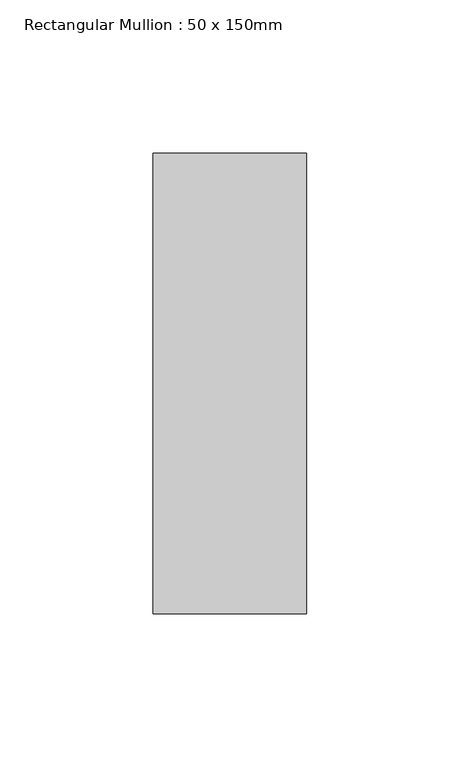
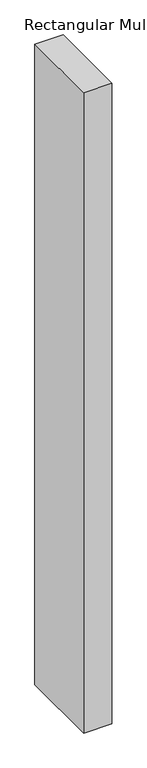
"""IFC4 building model written with IfcOpenShell, lengths in millimetres: member geometry, Rectangular Mullion : 50 x 150mm."""

from ifc_helpers import new_model, si_unit, frame, origin, place, context, project, spatial, polyline, outline, extrude, source, transform, mapped, element, save


def rectangular_mullion_50_x_150mm_6588f46c(model_context):
    return source(origin(), model_context, "Body", "SweptSolid", [
        extrude(outline(polyline([(0.0, 75.0), (0.0, -75.0), (-50.0, -75.0), (-50.0, 75.0), (0.0, 75.0)])), frame((0.0, 0.0, -1200.0), z_axis=(0.0, 0.0, 1.0), x_axis=(1.0, 0.0, 0.0)), (0.0, 0.0, 1.0), 1200.0),
    ])


if __name__ == "__main__":
    model = new_model("IFC4")
    model_context = context("Model", 3, world=origin())
    ifc_project = project(units=[si_unit("LENGTHUNIT", "METRE", prefix="MILLI")], contexts=[model_context])
    site = spatial("IfcSite", under=ifc_project)
    building = spatial("IfcBuilding", under=site)
    placement = place(None, origin())
    rectangular_mullion_50_x_150mm_shape = rectangular_mullion_50_x_150mm_6588f46c(model_context)
    element("IfcMember", 1, ObjectType="Rectangular Mullion : 50 x 150mm", at=placement, inside=building, context=model_context, shape_type="MappedRepresentation", body=[
        mapped(rectangular_mullion_50_x_150mm_shape, transform((0.0, 0.0, 0.0), x_axis=(1.0, 0.0, 0.0), y_axis=(0.0, 1.0, 0.0), z_axis=(0.0, 0.0, 1.0))),
    ])
    save(model, "model.ifc")

# Revit data of these elements
# Type "Rectangular Mullion : 50 x 150mm"
#   built-in parameter 1007304 = 0.492126 (stored number, unit not read)
#   built-in parameter 1007301 = 0.082021 (stored number, unit not read)
#   built-in parameter 1007300 = 0.082021 (stored number, unit not read)
# Element 1 (IfcMember, "Rectangular Mullion : 50 x 150mm")
#   Materials on its faces: "Aluminium"
# Materials
#   "Aluminium": class "Metal", colour RGB 247 247 247, transparency 0, Description = "Aluminium 6061", Cost = 0
